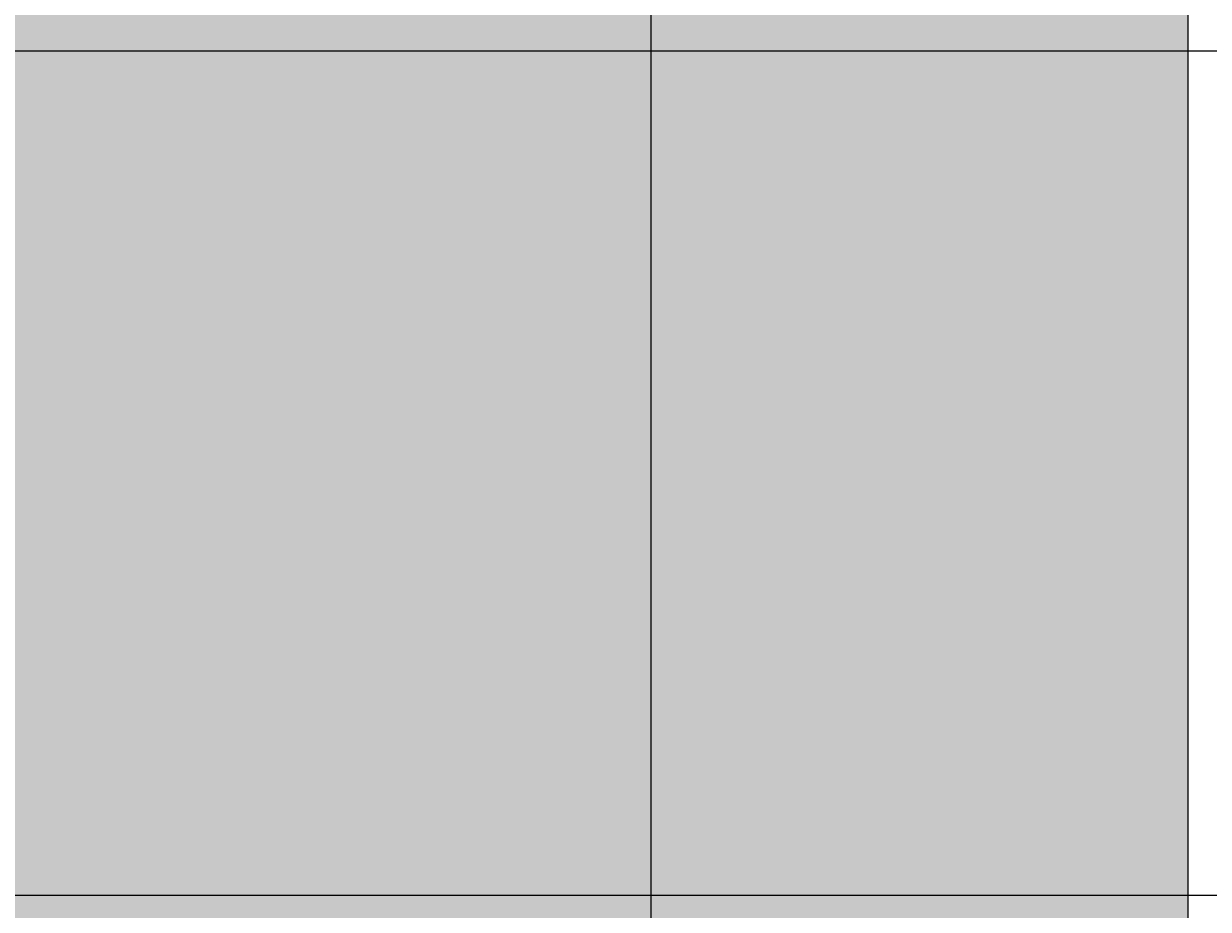
# Model space of a CAD drawing. Units: inches. Extents: x 35362 to 73946, y 43607 to 67532.
# Tile 66 of 134: x 47763 to 48170, y 48965 to 49269. Entities that reach past the tile are written whole.
import ezdxf

# ---------------------------------------------------------------- set-up
doc = ezdxf.new("R2010")
doc.units = ezdxf.units.IN
doc.header["$MEASUREMENT"] = 0
for name, color, linetype, lineweight in [('A-ANNO-DIMS', 2, 'Continuous', 18), ('E-SYMB', 1, 'Continuous', 25), ('E-SYMB-PATT', 1, 'Continuous', 13)]:
    doc.layers.add(name, color=color, linetype=linetype, lineweight=lineweight)
doc.styles.get("Standard").update_dxf_attribs({"font": 'arial.ttf'})
doc.dimstyles.get("Standard").update_dxf_attribs({"dimtxt": 0.18, "dimasz": 0.18, "dimexe": 0.18, "dimexo": 0.0625, "dimgap": 0.09, "dimtad": 0, "dimtih": 1, "dimtoh": 1, "dimdec": 4, "dimzin": 0, "dimdsep": 46, "dimtxsty": 'Standard', "dimcen": 0.09, "dimadec": 0, "dimazin": 0, "dimtfac": 1, "dimtdec": 4, "dimtofl": 0, "dimtmove": 0, "dimatfit": 3, "dimfxl": 1, "dimtolj": 1, "dimtzin": 0, "dimarcsym": 0})

# ---------------------------------------------------------------- blocks, each defined once
blk = doc.blocks.new('*D11')
at = {"layer": 'A-ANNO-DIMS', "color": 0, "lineweight": -2, "transparency": 16777216}
for p, q in [((47978.66, 56028.77), (47978.66, 43606.68)), ((53109.76, 56028.77), (53109.76, 43606.68)), ((47978.84, 43606.86), (50543.87, 43606.86)), ((53109.58, 43606.86), (50544.55, 43606.86))]:
    blk.add_line(p, q, dxfattribs=at)
at = {"layer": 'A-ANNO-DIMS', "color": 0, "transparency": 16777216}
for points in [[(47978.84, 43606.89), (47978.84, 43606.83), (47978.66, 43606.86)], [(53109.58, 43606.89), (53109.58, 43606.83), (53109.76, 43606.86)]]:
    blk.add_solid(points, dxfattribs=at)
at = {"layer": 'Defpoints', "color": 0, "transparency": 16777216}
for p in [(47978.66, 56028.84), (53109.76, 56028.84), (53109.76, 43606.86)]:
    blk.add_point(p, dxfattribs=at)
at = {"layer": 'A-ANNO-DIMS', "color": 0, "transparency": 16777216, "insert": (50544.21, 43606.86), "char_height": 0.18, "attachment_point": 5}
blk.add_mtext('\\A1;5131', dxfattribs=at)
blk = doc.blocks.new('*D27')
at = {"layer": 'A-ANNO-DIMS', "color": 0, "lineweight": -2, "transparency": 16777216}
for p, q in [((47978.66, 56028.77), (47978.66, 43606.68)), ((48373.49, 53428.96), (48373.49, 43606.68)), ((47978.84, 43606.86), (48175.68, 43606.86)), ((48373.31, 43606.86), (48176.47, 43606.86))]:
    blk.add_line(p, q, dxfattribs=at)
at = {"layer": 'A-ANNO-DIMS', "color": 0, "transparency": 16777216}
for points in [[(47978.84, 43606.89), (47978.84, 43606.83), (47978.66, 43606.86)], [(48373.31, 43606.89), (48373.31, 43606.83), (48373.49, 43606.86)]]:
    blk.add_solid(points, dxfattribs=at)
at = {"layer": 'Defpoints', "color": 0, "transparency": 16777216}
for p in [(47978.66, 56028.84), (48373.49, 53429.02), (48373.49, 43606.86)]:
    blk.add_point(p, dxfattribs=at)
at = {"layer": 'A-ANNO-DIMS', "color": 0, "transparency": 16777216, "insert": (48176.08, 43606.86), "char_height": 0.18, "attachment_point": 5}
blk.add_mtext('\\A1;394.8', dxfattribs=at)
blk = doc.blocks.new('*D67')
at = {"layer": 'A-ANNO-DIMS', "color": 0, "lineweight": -2, "transparency": 16777216}
for p, q in [((56873.54, 53351.53), (35361.77, 53351.53)), ((35361.95, 53351.35), (35361.95, 49400.89)), ((35361.95, 45450.07), (35361.95, 49400.53)), ((53793.58, 45449.89), (35361.77, 45449.89))]:
    blk.add_line(p, q, dxfattribs=at)
at = {"layer": 'A-ANNO-DIMS', "color": 0, "transparency": 16777216}
for points in [[(35361.92, 53351.35), (35361.98, 53351.35), (35361.95, 53351.53)], [(35361.92, 45450.07), (35361.98, 45450.07), (35361.95, 45449.89)]]:
    blk.add_solid(points, dxfattribs=at)
at = {"layer": 'Defpoints', "color": 0, "transparency": 16777216}
for p in [(35361.95, 53351.53), (56873.6, 53351.53), (53793.64, 45449.89)]:
    blk.add_point(p, dxfattribs=at)
at = {"layer": 'A-ANNO-DIMS', "color": 0, "transparency": 16777216, "insert": (35361.95, 49400.71), "char_height": 0.18, "attachment_point": 5}
blk.add_mtext('\\A1;7901.6', dxfattribs=at)
blk = doc.blocks.new('*D84')
at = {"layer": 'A-ANNO-DIMS', "color": 0, "lineweight": -2, "transparency": 16777216}
for p, q in [((55540.23, 49259.94), (35361.77, 49259.94)), ((35361.95, 49259.76), (35361.95, 49115.14)), ((35361.95, 48970.16), (35361.95, 49114.78)), ((55540.23, 48969.98), (35361.77, 48969.98))]:
    blk.add_line(p, q, dxfattribs=at)
at = {"layer": 'A-ANNO-DIMS', "color": 0, "transparency": 16777216}
for points in [[(35361.92, 49259.76), (35361.98, 49259.76), (35361.95, 49259.94)], [(35361.92, 48970.16), (35361.98, 48970.16), (35361.95, 48969.98)]]:
    blk.add_solid(points, dxfattribs=at)
at = {"layer": 'Defpoints', "color": 0, "transparency": 16777216}
for p in [(35361.95, 49259.94), (55540.3, 49259.94), (55540.3, 48969.98)]:
    blk.add_point(p, dxfattribs=at)
at = {"layer": 'A-ANNO-DIMS', "color": 0, "transparency": 16777216, "insert": (35361.95, 49114.96), "char_height": 0.18, "attachment_point": 5}
blk.add_mtext('\\A1;289.96', dxfattribs=at)
blk = doc.blocks.new('*D86')
at = {"layer": 'A-ANNO-DIMS', "color": 0, "lineweight": -2, "transparency": 16777216}
for p, q in [((51285.53, 49320.08), (35361.77, 49320.08)), ((35361.95, 49319.9), (35361.95, 49120.26)), ((35361.95, 48920.26), (35361.95, 49119.9)), ((51285.53, 48920.08), (35361.77, 48920.08))]:
    blk.add_line(p, q, dxfattribs=at)
at = {"layer": 'A-ANNO-DIMS', "color": 0, "transparency": 16777216}
for points in [[(35361.92, 49319.9), (35361.98, 49319.9), (35361.95, 49320.08)], [(35361.92, 48920.26), (35361.98, 48920.26), (35361.95, 48920.08)]]:
    blk.add_solid(points, dxfattribs=at)
at = {"layer": 'Defpoints', "color": 0, "transparency": 16777216}
for p in [(35361.95, 49320.08), (51285.59, 49320.08), (51285.59, 48920.08)]:
    blk.add_point(p, dxfattribs=at)
at = {"layer": 'A-ANNO-DIMS', "color": 0, "transparency": 16777216, "insert": (35361.95, 49120.08), "char_height": 0.18, "attachment_point": 5}
blk.add_mtext('\\A1;400.0', dxfattribs=at)

msp = doc.modelspace()

# ---------------------------------------------------------------- hatches: boundary and pattern name
at = {"layer": 'E-SYMB-PATT'}
h = msp.add_hatch(color=256, dxfattribs=at)
h.dxf.hatch_style = 1
h.paths.add_polyline_path([(48163.038, 49689.843), (45390.147, 49689.843), (45390.147, 46919.381), (48163.038, 46919.381)])

# ---------------------------------------------------------------- linework, layer by layer
at = {"layer": 'E-SYMB'}
msp.add_lwpolyline([(45390.147, 49689.843), (48163.038, 49689.843), (48163.038, 46919.381), (45390.147, 46919.381)], close=True, dxfattribs=at)

# ---------------------------------------------------------------- dimensions: what is measured, and where the dimension line sits
at = {"layer": 'A-ANNO-DIMS'}
for base, p2, override, picture, middle in [((53109.76, 43606.859), (53109.76, 56028.836), {"dimdec": 0, "dimlfac": 1, "dimrnd": 0, "dimzin": 0, "dimdsep": 46, "dimlunit": 2}, '*D11', (50544.212, 43606.859)), ((48373.492, 43606.859), (48373.492, 53429.019), {"dimdec": 1, "dimlfac": 1, "dimrnd": 0, "dimzin": 0, "dimdsep": 46, "dimlunit": 2}, '*D27', (48176.078, 43606.859))]:
    dim = msp.add_linear_dim(base=base, p1=(47978.665, 56028.836), p2=p2, dimstyle='Standard', override=override, dxfattribs=at)
    dim.commit()
    dim.dimension.update_dxf_attribs({"geometry": picture, "text_midpoint": middle})
for base, p1, p2, override, picture, middle in [((35361.949, 53351.529), (53793.638, 45449.894), (56873.602, 53351.529), {"dimdec": 1, "dimlfac": 1, "dimrnd": 0, "dimzin": 0, "dimdsep": 46, "dimlunit": 2}, '*D67', (35361.949, 49400.712)), ((35361.949, 49320.079), (51285.595, 48920.079), (51285.595, 49320.079), {"dimdec": 1, "dimlfac": 1, "dimrnd": 0, "dimzin": 0, "dimdsep": 46, "dimlunit": 2}, '*D86', (35361.949, 49120.079)), ((35361.9491, 49259.9353), (55540.2972, 48969.9796), (55540.2972, 49259.9353), {"dimdec": 2, "dimlfac": 1, "dimrnd": 0, "dimzin": 0, "dimdsep": 46, "dimlunit": 2}, '*D84', (35361.9491, 49114.9575))]:
    dim = msp.add_linear_dim(base=base, p1=p1, p2=p2, angle=90, dimstyle='Standard', override=override, dxfattribs=at)
    dim.commit()
    dim.dimension.update_dxf_attribs({"geometry": picture, "text_midpoint": middle})

doc.saveas('drawing.dxf')
